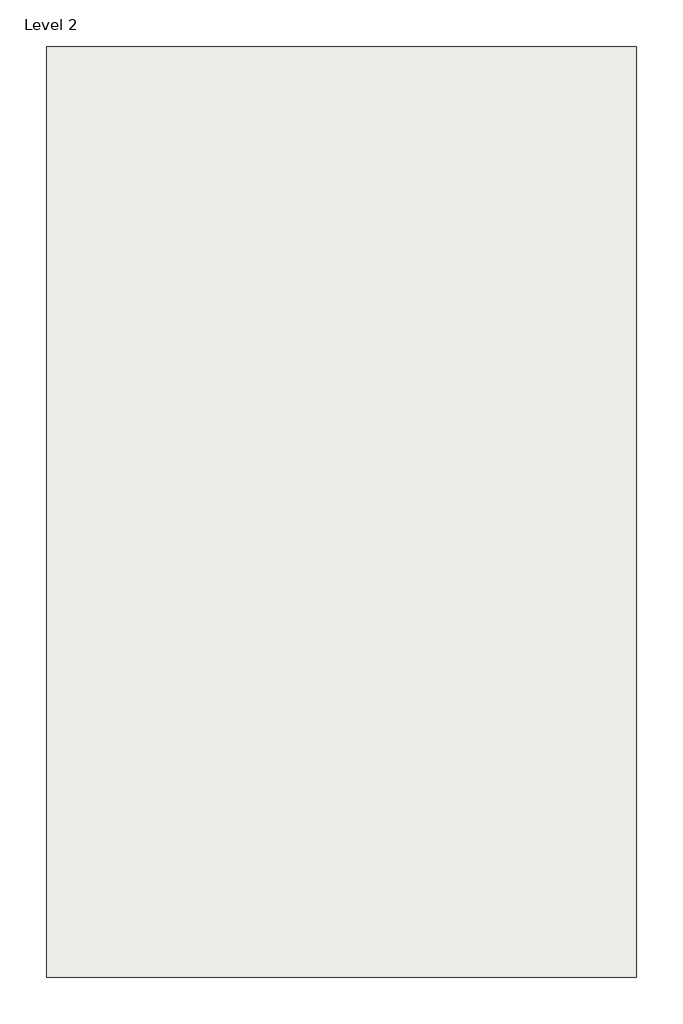
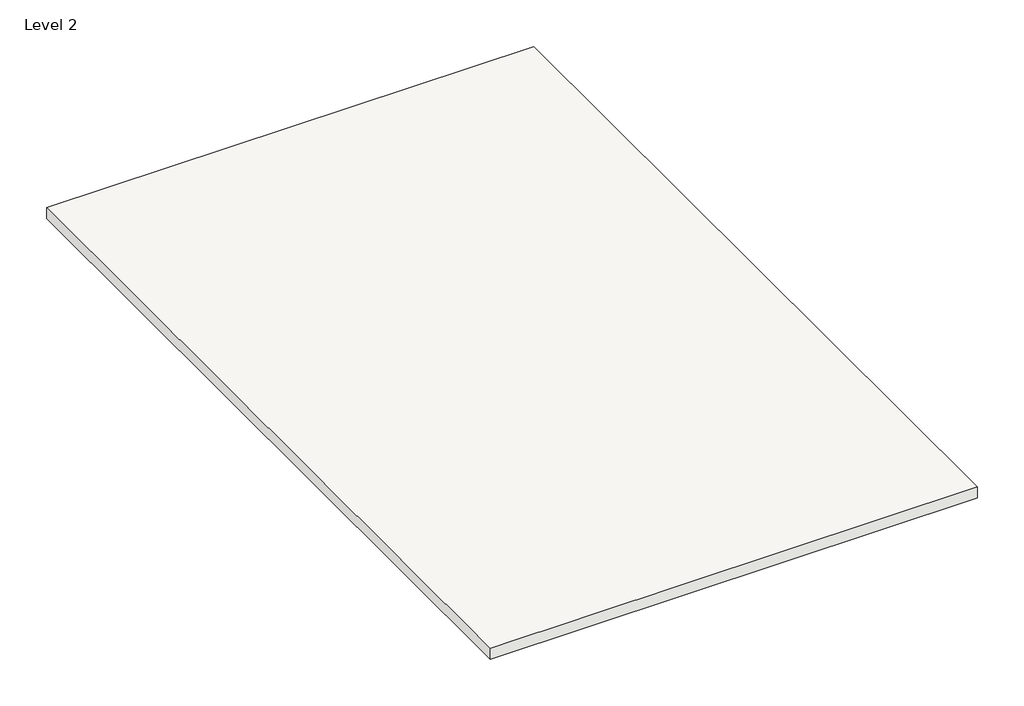
# One storey: 1 roof.
"""IFC4 building model written with IfcOpenShell, lengths in millimetres."""

from ifc_helpers import new_model, si_unit, frame, origin, place, context, project, spatial, polyline, outline, extrude, element, save

model = new_model("IFC4")

# Units and contexts
model_context = context("Model", 3, world=origin())
ifc_project = project(units=[si_unit("LENGTHUNIT", "METRE", prefix="MILLI")], contexts=[model_context])

# Site, building, storey
site = spatial("IfcSite", under=ifc_project)
building = spatial("IfcBuilding", under=site)
storey = spatial("IfcBuildingStorey", under=building, Name="Level 2", Elevation=3048.0)

# Roof
placement = place(None, origin())
element("IfcRoof", 1, ObjectType="Generic - 12\"", at=placement, inside=storey, context=model_context, shape_type="SweptSolid", body=[
    extrude(outline(polyline([(-11087.3357228, 14812.8620171), (1663.4642772, 14812.8620171), (1663.4642772, -5303.9379829), (-11087.3357228, -5303.9379829), (-11087.3357228, 14812.8620171)])), frame((0.0, 0.0, 3048.0), z_axis=(0.0, 0.0, 1.0), x_axis=(1.0, 0.0, 0.0)), (0.0, 0.0, 1.0), 304.8),
])

save(model, "model.ifc")

# Revit data of these elements
# Type "Generic - 12\""
#   Assembly Code = "B1020"
#   Layers, outside or top first: 1' - 0" "Brick, Soldier Course" (function 1)
# Element 1 (IfcRoof, "Generic - 12\"")
#   built-in parameter 1001705 = 11 (stored number, unit not read)
#   built-in parameter 1001710 = 33615
#   Phase Created = New Construction
#   Materials on its faces: "Brick, Soldier Course"
# Materials
#   "Brick, Soldier Course": class "Masonry", colour RGB 170 98 104, transparency 0, Description = "Common brick soldier coursed", Cost = 0
